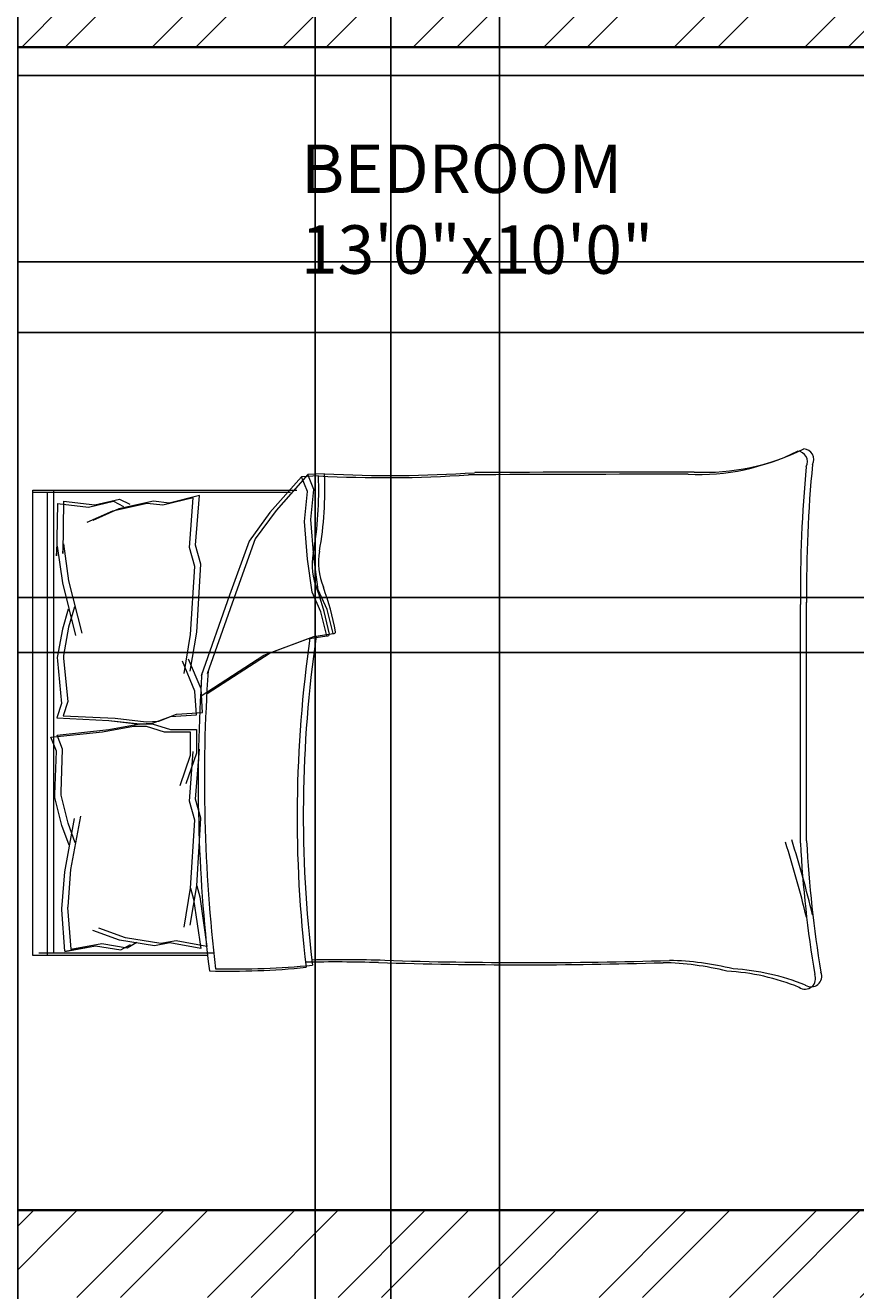
# Model space of a CAD drawing. Units: inches. Extents: x 1748 to 2382, y 1346 to 2284.
# Tile 19 of 26: x 1871 to 1956, y 1971 to 2102. Entities that reach past the tile are written whole.
import ezdxf

# ---------------------------------------------------------------- set-up
doc = ezdxf.new("R2010")
doc.units = ezdxf.units.IN
for name, color, linetype, lineweight in [('A-ANNO-DIMS', 2, 'Continuous', 18), ('A-AREA-IDEN', 7, 'Continuous', 18), ('A-FURN', 8, 'Continuous', 13), ('A-WALL', 7, 'Continuous', 35), ('A-WALL-PATT', 9, 'Continuous', 13)]:
    doc.layers.add(name, color=color, linetype=linetype, lineweight=lineweight)
doc.styles.get("Standard").update_dxf_attribs({"font": 'arial.ttf'})
doc.dimstyles.get("Standard").update_dxf_attribs({"dimtxt": 0.18, "dimasz": 0.18, "dimexe": 0.18, "dimexo": 0.0625, "dimgap": 0.09, "dimtad": 0, "dimtih": 1, "dimtoh": 1, "dimdec": 4, "dimzin": 0, "dimdsep": 46, "dimtxsty": 'Standard', "dimcen": 0.09, "dimadec": 0, "dimazin": 0, "dimtfac": 1, "dimtdec": 4, "dimtofl": 0, "dimtmove": 0, "dimatfit": 3, "dimfxl": 1, "dimtolj": 1, "dimtzin": 0, "dimarcsym": 0})

# ---------------------------------------------------------------- blocks, each defined once
blk = doc.blocks.new('BED-DOUBLE')
for p, q in [((3.48, 63.33), (3.48, 81.44)), ((3.48, 63.33), (3.48, 81.44)), ((3.48, 81.44), (51.49, 81.44)), ((51.27, 81.44), (51.27, 54.83)), ((51.27, 81.44), (51.27, 54.83)), ((51.49, 81.44), (51.49, 80.8)), ((3.48, 79.91), (51.27, 79.91)), ((3.48, 79.91), (51.27, 79.91)), ((3.7, 62.69), (3.7, 80.8)), ((3.7, 62.69), (3.7, 80.8)), ((51.49, 80.8), (51.49, 54.19)), ((51.49, 80.8), (51.49, 54.19)), ((3.7, 79.27), (51.49, 79.27)), ((3.7, 79.27), (51.49, 79.27)), ((3.9, 78.11), (8.18, 78.43)), ((3.9, 78.11), (8.18, 78.43)), ((8.18, 78.43), (8.29, 78.42)), ((8.18, 78.43), (8.28, 78.42)), ((8.28, 78.42), (12.11, 78.13)), ((8.29, 78.42), (12.11, 78.13)), ((14.86, 77.69), (16.88, 78.42)), ((14.86, 77.69), (16.88, 78.42)), ((16.88, 78.42), (19.77, 79.14)), ((16.88, 78.42), (19.77, 79.14)), ((17.11, 77.78), (20, 78.5)), ((17.11, 77.78), (20, 78.5)), ((19.77, 79.14), (20.09, 79.14)), ((19.77, 79.14), (20.09, 79.14)), ((20, 78.5), (20.32, 78.5)), ((20, 78.5), (20.32, 78.5)), ((20.09, 79.14), (24.54, 78.99)), ((20.09, 79.14), (24.54, 78.99)), ((20.32, 78.5), (24.77, 78.36)), ((20.32, 78.5), (24.77, 78.36)), ((24.54, 78.99), (25.98, 79.57)), ((24.54, 78.99), (25.98, 79.57)), ((24.77, 78.36), (26.21, 78.93)), ((24.77, 78.36), (26.21, 78.93)), ((25.98, 79.57), (26.56, 74.22)), ((25.98, 79.57), (26.56, 74.22)), ((26.21, 78.93), (26.79, 73.58)), ((26.21, 78.93), (26.79, 73.58)), ((27.98, 78.95), (27.73, 73.58)), ((27.98, 78.95), (27.73, 73.58)), ((29.46, 78.46), (27.98, 78.95)), ((29.46, 78.46), (27.98, 78.95)), ((33.88, 78.89), (29.46, 78.46)), ((33.88, 78.89), (29.46, 78.46)), ((34.21, 78.91), (33.88, 78.89)), ((34.2, 78.91), (33.88, 78.89)), ((37.14, 78.37), (34.2, 78.91)), ((37.14, 78.37), (34.21, 78.91)), ((41.91, 78.37), (36.5, 77.02)), ((41.91, 78.37), (36.5, 77.02)), ((39.2, 77.77), (37.14, 78.37)), ((39.2, 77.77), (37.14, 78.37)), ((45.71, 78.9), (41.91, 78.37)), ((45.71, 78.9), (41.91, 78.37)), ((50.11, 78.89), (44.71, 78.98)), ((44.71, 78.98), (45.71, 78.9)), ((50.11, 78.89), (44.71, 78.98)), ((44.71, 78.98), (45.71, 78.9)), ((50.34, 78.25), (44.94, 78.34)), ((44.94, 78.34), (45.94, 78.26)), ((50.34, 78.25), (44.94, 78.34)), ((44.94, 78.34), (45.94, 78.26)), ((50.11, 78.89), (49.73, 75.68)), ((50.11, 78.89), (49.73, 75.68)), ((3.89, 78.13), (4.47, 74.95)), ((3.9, 78.13), (4.47, 74.95)), ((4.12, 77.49), (4.7, 74.31)), ((4.12, 77.49), (4.7, 74.31)), ((4.13, 77.47), (8.41, 77.8)), ((4.13, 77.47), (8.41, 77.8)), ((8.41, 77.8), (8.51, 77.78)), ((8.41, 77.8), (8.51, 77.78)), ((8.51, 77.78), (12.34, 77.49)), ((8.51, 77.78), (12.34, 77.49)), ((12.11, 78.13), (17.6, 77.12)), ((12.11, 78.13), (17.6, 77.12)), ((12.34, 77.49), (17.83, 76.48)), ((12.34, 77.49), (17.83, 76.48)), ((15.08, 77.05), (17.11, 77.78)), ((15.08, 77.05), (17.11, 77.78)), ((28.21, 78.31), (27.96, 72.94)), ((28.21, 78.31), (27.96, 72.94)), ((29.68, 77.83), (28.21, 78.31)), ((29.68, 77.83), (28.21, 78.31)), ((34.11, 78.25), (29.68, 77.83)), ((34.11, 78.25), (29.68, 77.83)), ((34.43, 78.27), (34.11, 78.25)), ((34.43, 78.27), (34.11, 78.25)), ((37.36, 77.73), (34.43, 78.27)), ((37.36, 77.73), (34.43, 78.27)), ((42.14, 77.73), (36.72, 76.38)), ((42.14, 77.73), (36.72, 76.38)), ((39.43, 77.13), (37.36, 77.73)), ((39.43, 77.13), (37.36, 77.73)), ((45.94, 78.26), (42.14, 77.73)), ((45.94, 78.26), (42.14, 77.73)), ((50.34, 78.25), (49.96, 75.04)), ((50.34, 78.25), (49.96, 75.04)), ((49.31, 73.19), (48.13, 75.87)), ((49.31, 73.19), (48.13, 75.87)), ((4.47, 74.95), (4.04, 72.34)), ((4.47, 74.95), (4.04, 72.34)), ((5.05, 72.49), (6.06, 75.24)), ((5.05, 72.49), (6.06, 75.24)), ((5.28, 71.85), (6.29, 74.6)), ((5.28, 71.85), (6.29, 74.6)), ((49.54, 72.55), (48.36, 75.23)), ((49.54, 72.55), (48.36, 75.23)), ((49.73, 75.68), (50.33, 73.11)), ((49.73, 75.68), (50.33, 73.11)), ((49.96, 75.04), (50.56, 72.47)), ((49.96, 75.04), (50.56, 72.47)), ((4.7, 74.31), (4.27, 71.7)), ((4.7, 74.31), (4.27, 71.7)), ((26.56, 74.22), (27.14, 71.04)), ((26.56, 74.22), (27.14, 71.04)), ((26.79, 73.58), (27.37, 70.4)), ((26.79, 73.58), (27.37, 70.4)), ((27.73, 73.58), (27.35, 70.37)), ((27.73, 73.58), (27.36, 70.37)), ((50.11, 69.61), (49.31, 73.19)), ((50.11, 69.61), (49.31, 73.19)), ((4.04, 72.34), (4.62, 71.33)), ((4.04, 72.34), (4.62, 71.33)), ((4.47, 68.87), (5.05, 72.49)), ((4.47, 68.87), (5.05, 72.49)), ((4.7, 68.23), (5.28, 71.85)), ((4.7, 68.23), (5.28, 71.85)), ((27.96, 72.94), (27.58, 69.73)), ((27.96, 72.94), (27.58, 69.73)), ((50.34, 68.98), (49.54, 72.55)), ((50.34, 68.98), (49.54, 72.55)), ((50.33, 73.11), (49.81, 72.06)), ((50.33, 73.11), (49.81, 72.06)), ((50.56, 72.47), (50.04, 71.42)), ((50.56, 72.47), (50.04, 71.42)), ((4.27, 71.7), (4.85, 70.69)), ((4.27, 71.7), (4.85, 70.69)), ((27.14, 71.04), (27.14, 69.74)), ((27.14, 71.04), (27.14, 69.74)), ((27.14, 69.74), (26.56, 67.86)), ((27.14, 69.74), (26.56, 67.86)), ((27.35, 70.37), (27.44, 69.07)), ((27.36, 70.37), (27.44, 69.07)), ((27.37, 70.4), (27.37, 69.1)), ((27.37, 70.4), (27.37, 69.1)), ((27.58, 69.73), (27.66, 68.43)), ((27.58, 69.73), (27.66, 68.43)), ((49.92, 68.01), (50.11, 69.61)), ((49.92, 68.01), (50.11, 69.61)), ((4.76, 67.28), (4.47, 68.87)), ((4.76, 67.28), (4.47, 68.87)), ((4.99, 66.64), (4.7, 68.23)), ((4.99, 66.64), (4.7, 68.23)), ((27.37, 69.1), (26.79, 67.22)), ((27.37, 69.1), (26.79, 67.22)), ((27.44, 69.07), (28.13, 67.23)), ((27.44, 69.07), (28.13, 67.23)), ((27.66, 68.43), (28.36, 66.59)), ((27.66, 68.43), (28.36, 66.59)), ((50.7, 64.87), (49.92, 68.01)), ((50.7, 64.87), (49.92, 68.01)), ((50.15, 67.37), (50.34, 68.98)), ((50.15, 67.37), (50.34, 68.98)), ((4.18, 64.1), (4.76, 67.28)), ((4.18, 64.1), (4.76, 67.28)), ((4.41, 63.46), (4.99, 66.64)), ((4.41, 63.46), (4.99, 66.64)), ((26.56, 67.86), (26.56, 65.18)), ((26.56, 67.86), (26.56, 65.18)), ((26.79, 67.22), (26.79, 64.54)), ((26.79, 67.22), (26.79, 64.54)), ((28.13, 67.23), (28.3, 64.55)), ((28.13, 67.23), (28.3, 64.55)), ((28.36, 66.59), (28.53, 63.91)), ((28.36, 66.59), (28.53, 63.91)), ((50.93, 64.23), (50.15, 67.37)), ((50.93, 64.23), (50.15, 67.37)), ((6.38, 65.81), (10.41, 65.15)), ((6.38, 65.81), (10.41, 65.15)), ((24.1, 65.18), (20.96, 66.27)), ((24.1, 65.18), (20.96, 66.27)), ((24.33, 64.54), (21.19, 65.63)), ((24.33, 64.54), (21.19, 65.63)), ((30.75, 64.7), (33.82, 65.99)), ((30.75, 64.7), (33.82, 65.99)), ((30.98, 64.06), (34.05, 65.35)), ((30.98, 64.06), (34.05, 65.35)), ((32.56, 65.81), (36.6, 65.15)), ((32.56, 65.81), (36.6, 65.15)), ((9.28, 64.83), (4.18, 64.1)), ((9.28, 64.83), (4.18, 64.1)), ((9.51, 64.19), (4.41, 63.46)), ((9.51, 64.19), (4.41, 63.46)), ((6.61, 65.18), (10.64, 64.51)), ((6.61, 65.18), (10.64, 64.51)), ((10.41, 65.15), (9.28, 64.83)), ((10.41, 65.15), (9.28, 64.83)), ((10.64, 64.51), (9.51, 64.19)), ((10.64, 64.51), (9.51, 64.19)), ((10.41, 65.15), (17.42, 64.72)), ((10.41, 65.15), (17.42, 64.72)), ((10.64, 64.51), (17.65, 64.08)), ((10.64, 64.51), (17.65, 64.08)), ((17.42, 64.72), (19.38, 65.27)), ((17.42, 64.72), (19.38, 65.27)), ((17.65, 64.08), (19.61, 64.64)), ((17.65, 64.08), (19.61, 64.64)), ((19.38, 65.27), (24.52, 64.87)), ((19.38, 65.27), (24.52, 64.87)), ((19.61, 64.64), (24.74, 64.23)), ((19.61, 64.64), (24.74, 64.23)), ((26.56, 65.18), (24.1, 65.18)), ((26.56, 65.18), (24.1, 65.18)), ((26.79, 64.54), (24.33, 64.54)), ((26.79, 64.54), (24.33, 64.54)), ((28.3, 64.55), (30.75, 64.7)), ((28.3, 64.55), (30.75, 64.7)), ((28.53, 63.91), (30.98, 64.06)), ((28.53, 63.91), (30.98, 64.06)), ((30.26, 64.06), (34.45, 57.57)), ((30.26, 64.06), (34.45, 57.57)), ((40.64, 61.13), (32.31, 64.06)), ((40.64, 61.13), (32.31, 64.06)), ((32.79, 65.18), (36.83, 64.51)), ((32.79, 65.18), (36.82, 64.51)), ((36.6, 65.15), (43.61, 64.72)), ((36.6, 65.15), (43.61, 64.72)), ((36.82, 64.51), (43.83, 64.08)), ((36.83, 64.51), (43.83, 64.08)), ((43.61, 64.72), (45.57, 65.27)), ((43.61, 64.72), (45.57, 65.27)), ((43.83, 64.08), (45.8, 64.64)), ((43.83, 64.08), (45.79, 64.64)), ((45.57, 65.27), (50.7, 64.87)), ((45.57, 65.27), (50.7, 64.87)), ((45.79, 64.64), (50.93, 64.23)), ((45.8, 64.64), (50.93, 64.23)), ((30.49, 63.42), (34.68, 56.93)), ((30.49, 63.42), (34.68, 56.93)), ((40.87, 60.49), (32.53, 63.42)), ((40.87, 60.49), (32.53, 63.42)), ((46.22, 59.11), (40.64, 61.13)), ((46.22, 59.11), (40.64, 61.13)), ((46.45, 58.48), (40.87, 60.49)), ((46.45, 58.48), (40.87, 60.49)), ((49.16, 56.95), (46.22, 59.11)), ((49.16, 56.95), (46.22, 59.11)), ((34.45, 57.57), (36.15, 53.08)), ((34.45, 57.57), (36.15, 53.08)), ((49.39, 56.31), (46.45, 58.48)), ((49.39, 56.31), (46.45, 58.48)), ((34.68, 56.93), (36.38, 52.44)), ((34.68, 56.93), (36.38, 52.44)), ((52.87, 53.7), (49.16, 56.95)), ((52.87, 53.7), (49.16, 56.95)), ((53.1, 53.06), (49.39, 56.31)), ((53.1, 53.06), (49.39, 56.31)), ((51.33, 53.08), (52.87, 53.7)), ((51.33, 53.08), (52.87, 53.7)), ((52.95, 51.95), (52.87, 53.7, 3.87)), ((52.95, 51.95), (52.87, 53.7, 3.87)), ((36.15, 53.08), (36.46, 51.07)), ((36.15, 53.08), (36.46, 51.07)), ((36.38, 52.44), (36.69, 50.43)), ((36.38, 52.44), (36.69, 50.43)), ((38.94, 51.69), (40.95, 52.61)), ((38.94, 51.69), (40.95, 52.61)), ((40.95, 52.61), (44.36, 53.08)), ((40.95, 52.61), (44.36, 53.08)), ((41.18, 51.97), (44.59, 52.44)), ((41.18, 51.97), (44.59, 52.44)), ((44.36, 53.08), (48.23, 53.39)), ((44.36, 53.08), (48.23, 53.39)), ((44.59, 52.44), (48.46, 52.75)), ((44.59, 52.44), (48.46, 52.75)), ((48.23, 53.39), (51.33, 53.08)), ((48.23, 53.39), (51.33, 53.08)), ((48.46, 52.75), (51.56, 52.44)), ((48.46, 52.75), (51.56, 52.44)), ((51.56, 52.44), (53.1, 53.06)), ((51.56, 52.44), (53.1, 53.06)), ((53.18, 51.31), (53.1, 53.06, 3.87)), ((53.18, 51.31), (53.1, 53.06, 3.87)), ((36.46, 51.07), (38.94, 51.69)), ((36.46, 51.07), (38.94, 51.69)), ((36.69, 50.43), (39.17, 51.05)), ((36.69, 50.43), (39.17, 51.05)), ((39.17, 51.05), (41.18, 51.97)), ((39.17, 51.05), (41.18, 51.97)), ((15.06, 2.2), (39.68, 2.2)), ((15.06, 2.2), (39.68, 2.2)), ((15.29, 1.56), (39.91, 1.56)), ((15.29, 1.56), (39.91, 1.56))]:
    blk.add_line(p, q)
for centre, radius, start, end in [((21.36, -100.61), 164.97, 86.0865, 96.7821), ((21.36, -100.61), 164.97, 86.0865, 96.7821), ((85.16, 61.35), 83.31, 178.7218, 185.604), ((85.16, 61.35), 83.31, 178.7218, 185.604), ((21.59, -101.25), 164.97, 86.0865, 96.7821), ((21.59, -101.25), 164.97, 86.0865, 96.7821), ((85.39, 60.71), 83.31, 178.7218, 185.604), ((85.39, 60.71), 83.31, 178.7218, 185.604), ((17.76, -74.87), 129.02, 81.7845, 96.9006), ((17.76, -74.87), 129.02, 81.7845, 96.9006), ((17.98, -75.51), 129.02, 81.7845, 96.9006), ((17.98, -75.51), 129.02, 81.7845, 96.9006), ((-167.31, 50.27), 170.11, 358.4762, 1.0082), ((-167.31, 50.27), 170.11, 358.4762, 1.0082), ((-167.08, 49.63), 170.11, 358.4762, 1.0082), ((-167.08, 49.63), 170.11, 358.4762, 1.0082), ((43.74, 46.38), 6.22, 78.6608, 113.7384), ((43.74, 46.38), 6.22, 78.6608, 113.7384), ((51.33, 88.1), 36.18, 259.8763, 272.5657), ((51.33, 88.1), 36.18, 259.8763, 272.5657), ((36.64, 51), 0.185, 160.2464, 271.1377), ((36.64, 51), 0.185, 160.2464, 271.1377), ((31.15, 79.96), 29.65, 280.6617, 289.8806), ((31.15, 79.96), 29.65, 280.6617, 289.8806), ((31.38, 79.32), 29.65, 280.6617, 289.8806), ((31.38, 79.32), 29.65, 280.6617, 289.8806), ((43.97, 45.74), 6.22, 78.6608, 113.7384), ((43.97, 45.74), 6.22, 78.6608, 113.7384), ((51.56, 87.46), 36.18, 259.8763, 272.5657), ((51.56, 87.46), 36.18, 259.8763, 272.5657), ((182.27, 45.13), 129.5, 176.9791, 183.8365), ((182.27, 45.13), 129.5, 176.9791, 183.8365), ((182.49, 44.49), 129.5, 176.9791, 183.8365), ((182.49, 44.49), 129.5, 176.9791, 183.8365), ((36.87, 50.36), 0.185, 160.2464, 271.1377), ((36.86, 50.36), 0.185, 160.2464, 271.1377), ((484.82, 30.83), 482.31, 178.2277, 181.7185), ((484.82, 30.83), 482.31, 178.2277, 181.7185), ((485.05, 30.19), 482.31, 178.2277, 181.7185), ((485.05, 30.19), 482.31, 178.2277, 181.7185), ((-4508.74, 13.62), 4561.86, 0.00217, 0.28689), ((-4508.74, 13.62), 4561.86, 0.00217, 0.28689), ((-4508.51, 12.98), 4561.86, 0.00217, 0.28689), ((-4508.51, 12.98), 4561.86, 0.00217, 0.28689), ((-26.9, 16.93), 29.63, 346.0648, 358.9113), ((-26.9, 16.93), 29.63, 346.0648, 358.9113), ((-26.67, 16.29), 29.63, 346.0648, 358.9113), ((-26.67, 16.29), 29.63, 346.0648, 358.9113), ((76.16, 12.78), 23.07, 177.4714, 206.4681), ((76.16, 12.78), 23.07, 177.4714, 206.4681), ((76.39, 12.14), 23.07, 177.4714, 206.4681), ((76.39, 12.14), 23.07, 177.4714, 206.4681), ((-21.66, 11.17), 23.56, 337.9751, 356.652), ((-21.66, 11.17), 23.56, 337.9751, 356.652), ((-21.43, 10.53), 23.56, 337.9751, 356.652), ((-21.43, 10.53), 23.56, 337.9751, 356.652), ((-17.22, 105.16), 106.46, 283.3832, 287.7053), ((-17.22, 105.16), 106.46, 283.3832, 287.7053), ((-16.99, 104.52), 106.46, 283.3832, 287.7053), ((-16.99, 104.52), 106.46, 283.3832, 287.7053), ((1.09, 1.73), 1.09, 146.1736, 293.4781), ((1.09, 1.73), 1.09, 146.1736, 293.4781), ((1.32, 1.09), 1.09, 146.1736, 293.4781), ((1.32, 1.09), 1.09, 146.1736, 293.4781), ((21.43, -119.39), 121.76, 92.9958, 99.4091), ((21.43, -119.39), 121.76, 92.9958, 99.4091), ((21.66, -120.03), 121.76, 92.9958, 99.4091), ((21.66, -120.03), 121.76, 92.9958, 99.4091), ((41.15, -130.83), 133.04, 84.4998, 90.6351), ((41.15, -130.83), 133.04, 84.4998, 90.6351), ((41.38, -131.47), 133.04, 84.4998, 90.6351), ((41.38, -131.47), 133.04, 84.4998, 90.6351), ((54.41, 2.57), 1.1, 242.6588, 356.02), ((54.41, 2.57), 1.1, 242.6588, 356.02), ((54.64, 1.93), 1.1, 242.6588, 356.02), ((54.64, 1.93), 1.1, 242.6588, 356.02)]:
    blk.add_arc(centre, radius, start, end)
blk = doc.blocks.new('*D50')
at = {"layer": 'A-ANNO-DIMS', "color": 0, "lineweight": -2, "transparency": 16777216}
for p, q in [((1869.96, 2223.79), (1869.96, 1360.47)), ((1908.44, 2223.79), (1908.44, 1360.47)), ((1870.14, 1360.65), (1888.81, 1360.65)), ((1908.26, 1360.65), (1889.6, 1360.65))]:
    blk.add_line(p, q, dxfattribs=at)
at = {"layer": 'A-ANNO-DIMS', "color": 0, "transparency": 16777216}
for points in [[(1870.14, 1360.68), (1870.14, 1360.62), (1869.96, 1360.65)], [(1908.26, 1360.68), (1908.26, 1360.62), (1908.44, 1360.65)]]:
    blk.add_solid(points, dxfattribs=at)
at = {"layer": 'Defpoints', "color": 0, "transparency": 16777216}
for p in [(1869.96, 2223.85), (1908.44, 2223.85), (1908.44, 1360.65)]:
    blk.add_point(p, dxfattribs=at)
at = {"layer": 'A-ANNO-DIMS', "color": 0, "transparency": 16777216, "insert": (1889.2, 1360.65), "char_height": 0.18, "attachment_point": 5}
blk.add_mtext('\\A1;38.48', dxfattribs=at)
blk = doc.blocks.new('*D57')
at = {"layer": 'A-ANNO-DIMS', "color": 0, "lineweight": -2, "transparency": 16777216}
for p, q in [((2288.4, 2099.35), (1779.88, 2099.35)), ((1780.06, 2099.17), (1780.06, 2088.46)), ((1780.06, 2077.38), (1780.06, 2088.09)), ((2288.4, 2077.2), (1779.88, 2077.2))]:
    blk.add_line(p, q, dxfattribs=at)
at = {"layer": 'A-ANNO-DIMS', "color": 0, "transparency": 16777216}
for points in [[(1780.03, 2099.17), (1780.09, 2099.17), (1780.06, 2099.35)], [(1780.03, 2077.38), (1780.09, 2077.38), (1780.06, 2077.2)]]:
    blk.add_solid(points, dxfattribs=at)
at = {"layer": 'Defpoints', "color": 0, "transparency": 16777216}
for p in [(1780.06, 2099.35), (2288.46, 2099.35), (2288.46, 2077.2)]:
    blk.add_point(p, dxfattribs=at)
at = {"layer": 'A-ANNO-DIMS', "color": 0, "transparency": 16777216, "insert": (1780.06, 2088.28), "char_height": 0.18, "attachment_point": 5}
blk.add_mtext('\\A1;22.15', dxfattribs=at)
blk = doc.blocks.new('*D63')
at = {"layer": 'A-ANNO-DIMS', "color": 0, "lineweight": -2, "transparency": 16777216}
for p, q in [((2253.72, 2042.57), (1779.88, 2042.57)), ((1780.06, 2042.39), (1780.06, 2039.92)), ((1780.06, 2037.08), (1780.06, 2039.55)), ((2253.72, 2036.9), (1779.88, 2036.9))]:
    blk.add_line(p, q, dxfattribs=at)
at = {"layer": 'A-ANNO-DIMS', "color": 0, "transparency": 16777216}
for points in [[(1780.03, 2042.39), (1780.09, 2042.39), (1780.06, 2042.57)], [(1780.03, 2037.08), (1780.09, 2037.08), (1780.06, 2036.9)]]:
    blk.add_solid(points, dxfattribs=at)
at = {"layer": 'Defpoints', "color": 0, "transparency": 16777216}
for p in [(1780.06, 2042.57), (2253.78, 2042.57), (2253.78, 2036.9)]:
    blk.add_point(p, dxfattribs=at)
at = {"layer": 'A-ANNO-DIMS', "color": 0, "transparency": 16777216, "insert": (1780.06, 2039.74), "char_height": 0.18, "attachment_point": 5}
blk.add_mtext('\\A1;5.673', dxfattribs=at)
blk = doc.blocks.new('*D64')
at = {"layer": 'A-ANNO-DIMS', "color": 0, "lineweight": -2, "transparency": 16777216}
for p, q in [((1900.64, 1476.91), (1900.64, 2274.93)), ((1900.82, 2274.75), (1909.7, 2274.75)), ((1919.5, 2274.75), (1910.62, 2274.75)), ((1919.68, 1476.91), (1919.68, 2274.93))]:
    blk.add_line(p, q, dxfattribs=at)
at = {"layer": 'A-ANNO-DIMS', "color": 0, "transparency": 16777216}
for points in [[(1900.82, 2274.78), (1900.82, 2274.72), (1900.64, 2274.75)], [(1919.5, 2274.78), (1919.5, 2274.72), (1919.68, 2274.75)]]:
    blk.add_solid(points, dxfattribs=at)
at = {"layer": 'Defpoints', "color": 0, "transparency": 16777216}
for p in [(1919.68, 2274.75), (1900.64, 1476.85), (1919.68, 1476.85)]:
    blk.add_point(p, dxfattribs=at)
at = {"layer": 'A-ANNO-DIMS', "color": 0, "transparency": 16777216, "insert": (1910.16, 2274.75), "char_height": 0.18, "attachment_point": 5}
blk.add_mtext('\\A1;19.035', dxfattribs=at)
blk = doc.blocks.new('*D76')
at = {"layer": 'A-ANNO-DIMS', "color": 0, "lineweight": -2, "transparency": 16777216}
for p, q in [((2025.9, 2096.43), (1779.88, 2096.43)), ((1780.06, 2096.25), (1780.06, 2083.35)), ((1780.06, 2070.08), (1780.06, 2082.98)), ((2025.9, 2069.9), (1779.88, 2069.9))]:
    blk.add_line(p, q, dxfattribs=at)
at = {"layer": 'A-ANNO-DIMS', "color": 0, "transparency": 16777216}
for points in [[(1780.03, 2096.25), (1780.09, 2096.25), (1780.06, 2096.43)], [(1780.03, 2070.08), (1780.09, 2070.08), (1780.06, 2069.9)]]:
    blk.add_solid(points, dxfattribs=at)
at = {"layer": 'Defpoints', "color": 0, "transparency": 16777216}
for p in [(1780.06, 2096.43), (2025.96, 2096.43), (2025.96, 2069.9)]:
    blk.add_point(p, dxfattribs=at)
at = {"layer": 'A-ANNO-DIMS', "color": 0, "transparency": 16777216, "insert": (1780.06, 2083.16), "char_height": 0.18, "attachment_point": 5}
blk.add_mtext('\\A1;26.535', dxfattribs=at)

msp = doc.modelspace()

# ---------------------------------------------------------------- hatches: boundary and pattern name
at = {"layer": 'A-WALL-PATT'}
h = msp.add_hatch(dxfattribs=at)
h.set_pattern_fill('ANSI32', color=256)
h.paths.add_polyline_path([(1908.4445, 2232.8497), (1821.9607, 2232.8497), (1821.9607, 2223.8497), (1865.4607, 2223.8497), (1865.4607, 2209.9185), (1869.9607, 2209.9185), (1869.9607, 2223.8497), (1908.4445, 2223.8497), (1908.4445, 2228.3497)])
h.paths.add_polyline_path([(2040.0683, 2232.8497), (1968.4445, 2232.8497), (1968.4445, 2223.8497), (2025.9607, 2223.8497), (2025.9607, 2130.3497), (2032.1341, 2130.3497), (2032.1341, 2132.5997), (2032.1341, 2134.8497), (2030.4607, 2134.8497), (2030.4607, 2223.8497), (2040.0683, 2223.8497)])
h.paths.add_polyline_path([(2091.3969, 2232.8497), (2064.0683, 2232.8497), (2064.0683, 2223.8497), (2078.4607, 2223.8497), (2078.4607, 2134.8497), (2051.1563, 2134.8497), (2051.1563, 2130.3497), (2078.4607, 2130.3497), (2078.4607, 2128.6813), (2082.9607, 2128.6813), (2082.9607, 2130.3497), (2086.1879, 2130.3497), (2086.1879, 2132.5997), (2086.1879, 2134.8497), (2082.9607, 2134.8497), (2082.9607, 2223.8497), (2091.3969, 2223.8497), (2091.3969, 2228.3497)])
h.paths.add_polyline_path([(2167.0164, 2232.8497), (2115.3969, 2232.8497), (2115.3969, 2223.8497), (2130.9607, 2223.8497), (2130.9607, 2134.8497), (2106.9607, 2134.8497), (2106.9607, 2130.3497), (2135.4607, 2130.3497), (2135.4607, 2223.8497), (2167.0164, 2223.8497), (2167.0164, 2228.3497)])
h.paths.add_polyline_path([(1869.9607, 2149.9185), (1865.4607, 2149.9185), (1865.4607, 2127.8942), (1869.9607, 2127.8942)])
h.paths.add_polyline_path([(2082.9607, 2104.4871), (2080.7107, 2104.4871), (2078.4607, 2104.4871), (2078.4607, 2103.8497), (1869.9607, 2103.8497), (1869.9607, 2108.6062), (1867.7107, 2108.6062), (1865.4607, 2108.6062), (1865.4607, 2103.8497), (1821.9607, 2103.8497), (1821.9607, 2099.3497), (1865.4607, 2099.3497), (1865.4607, 2094.7509), (1869.9607, 2094.7509), (1869.9607, 2099.3497), (2025.9607, 2099.3497), (2025.9607, 2096.4326), (2030.4607, 2096.4326), (2030.4607, 2099.3497), (2082.9607, 2099.3497)])
h.paths.add_polyline_path([(1928.9457, 1401.1212), (2176.8693, 1401.1212), (2176.8693, 1438.214), (1928.9457, 1438.214)], flags=9)
h.paths.add_polyline_path([(2122.2668, 2048.1927), (2177.9387, 2048.1927), (2177.9387, 2066.85), (2122.2668, 2066.85)], flags=9)
h.paths.add_polyline_path([(2272.688, 2153.8197), (2272.688, 2216.746), (2262.3845, 2216.746), (2262.3845, 2153.8197)], flags=9)
h.paths.add_polyline_path([(2157.2928, 2166.5593), (2196.3822, 2166.5593), (2196.3822, 2185.2167), (2157.2928, 2185.2167)], flags=9)
h.paths.add_polyline_path([(2089.3407, 2162.0698), (2124.3987, 2162.0698), (2124.3987, 2180.7272), (2089.3407, 2180.7272)], flags=9)
h.paths.add_polyline_path([(2037.4521, 2160.0913), (2072.5101, 2160.0913), (2072.5101, 2178.7486), (2037.4521, 2178.7486)], flags=9)
h.paths.add_polyline_path([(1884.7894, 2104.1554), (1923.6297, 2104.1554), (1923.6297, 2122.8127), (1884.7894, 2122.8127)], flags=9)
h.paths.add_polyline_path([(1851.2832, 2142.9749), (1851.2832, 2199.3051), (1840.9796, 2199.3051), (1840.9796, 2142.9749)], flags=9)
h.paths.add_polyline_path([(1844.8763, 2017.2834), (1844.8763, 2073.6136), (1834.5728, 2073.6136), (1834.5728, 2017.2834)], flags=9)
h.paths.add_polyline_path([(1897.1577, 2073.1279), (1935.9981, 2073.1279), (1935.9981, 2091.7853), (1897.1577, 2091.7853)], flags=9)
h.paths.add_polyline_path([(1952.3395, 1802.4231), (2008.0114, 1802.4231), (2008.0114, 1821.0805), (1952.3395, 1821.0805)], flags=9)
h.paths.add_polyline_path([(1978.8184, 1857.6841), (2017.7338, 1857.6841), (2017.7338, 1876.3415), (1978.8184, 1876.3415)], flags=9)
h.paths.add_polyline_path([(1979.6513, 1925.9516), (2008.8089, 1925.9516), (2008.8089, 1944.6089), (1979.6513, 1944.6089)], flags=9)
h.paths.add_polyline_path([(1838.5553, 1860.3527), (1877.3957, 1860.3527), (1877.3957, 1879.01), (1838.5553, 1879.01)], flags=9)
h.paths.add_polyline_path([(1883.9018, 1787.3013), (1883.9018, 1843.6315), (1873.5983, 1843.6315), (1873.5983, 1787.3013)], flags=9)
h.paths.add_polyline_path([(1873.7079, 1509.1938), (1873.7079, 1583.7709), (1863.4044, 1583.7709), (1863.4044, 1509.1938)], flags=9)
h.paths.add_polyline_path([(1916.2259, 1603.3681), (1955.0663, 1603.3681), (1955.0663, 1622.0254), (1916.2259, 1622.0254)], flags=9)
h.paths.add_polyline_path([(1876.3013, 1636.757), (1876.3013, 1693.0871), (1865.9978, 1693.0871), (1865.9978, 1636.757)], flags=9)
h.paths.add_polyline_path([(1921.3138, 1521.8316), (1964.0662, 1521.8316), (1964.0662, 1540.489), (1921.3138, 1540.489)], flags=9)
h.paths.add_polyline_path([(2017.5657, 1497.5078), (2046.7983, 1497.5078), (2046.7983, 1516.1651), (2017.5657, 1516.1651)], flags=9)
h.paths.add_polyline_path([(2066.8661, 1499.3902), (2096.0988, 1499.3902), (2096.0988, 1518.0475), (2066.8661, 1518.0475)], flags=9)
h.paths.add_polyline_path([(2155.4835, 1571.6596), (2198.2358, 1571.6596), (2198.2358, 1590.3169), (2155.4835, 1590.3169)], flags=9)
h.paths.add_polyline_path([(2094.9136, 1664.6812), (2150.5855, 1664.6812), (2150.5855, 1683.3386), (2094.9136, 1683.3386)], flags=9)
h.paths.add_polyline_path([(2257.6902, 1863.1628), (2269.8935, 1863.1628), (2269.8935, 1873.4664), (2257.6902, 1873.4664)], flags=9)
h.paths.add_polyline_path([(2164.0748, 1880.3089), (2189.8694, 1880.3089), (2189.8694, 1890.6124), (2164.0748, 1890.6124)], flags=9)
h.paths.add_polyline_path([(2239.4394, 1931.0585), (2268.8187, 1931.0585), (2268.8187, 1949.7159), (2239.4394, 1949.7159)], flags=9)
h = msp.add_hatch(dxfattribs=at)
h.set_pattern_fill('ANSI32', color=256)
h.paths.add_polyline_path([(2297.4607, 2232.8497), (2203.0164, 2232.8497), (2203.0164, 2223.8497), (2244.9607, 2223.8497), (2244.9607, 2127.8554), (2249.4607, 2127.8554), (2249.4607, 2223.8497), (2297.4607, 2223.8497)])
h.paths.add_polyline_path([(2297.4607, 2103.8497), (2249.4607, 2103.8497), (2249.4607, 2106.7497), (2247.2107, 2106.7497), (2244.9607, 2106.7497), (2244.9607, 2103.8497), (2130.9607, 2103.8497), (2130.9607, 2099.3497), (2288.4607, 2099.3497), (2288.4607, 2077.2008), (2297.4607, 2077.2008)])
h.paths.add_polyline_path([(1928.9457, 1401.1212), (2176.8693, 1401.1212), (2176.8693, 1438.214), (1928.9457, 1438.214)], flags=9)
h.paths.add_polyline_path([(2122.2668, 2048.1927), (2177.9387, 2048.1927), (2177.9387, 2066.85), (2122.2668, 2066.85)], flags=9)
h.paths.add_polyline_path([(2272.688, 2153.8197), (2272.688, 2216.746), (2262.3845, 2216.746), (2262.3845, 2153.8197)], flags=25)
h.paths.add_polyline_path([(2157.2928, 2166.5593), (2196.3822, 2166.5593), (2196.3822, 2185.2167), (2157.2928, 2185.2167)], flags=9)
h.paths.add_polyline_path([(2089.3407, 2162.0698), (2124.3987, 2162.0698), (2124.3987, 2180.7272), (2089.3407, 2180.7272)], flags=9)
h.paths.add_polyline_path([(2037.4521, 2160.0913), (2072.5101, 2160.0913), (2072.5101, 2178.7486), (2037.4521, 2178.7486)], flags=9)
h.paths.add_polyline_path([(1884.7894, 2104.1554), (1923.6297, 2104.1554), (1923.6297, 2122.8127), (1884.7894, 2122.8127)], flags=9)
h.paths.add_polyline_path([(1851.2832, 2142.9749), (1851.2832, 2199.3051), (1840.9796, 2199.3051), (1840.9796, 2142.9749)], flags=9)
h.paths.add_polyline_path([(1844.8763, 2017.2834), (1844.8763, 2073.6136), (1834.5728, 2073.6136), (1834.5728, 2017.2834)], flags=9)
h.paths.add_polyline_path([(1897.1577, 2073.1279), (1935.9981, 2073.1279), (1935.9981, 2091.7853), (1897.1577, 2091.7853)], flags=9)
h.paths.add_polyline_path([(1952.3395, 1802.4231), (2008.0114, 1802.4231), (2008.0114, 1821.0805), (1952.3395, 1821.0805)], flags=9)
h.paths.add_polyline_path([(1978.8184, 1857.6841), (2017.7338, 1857.6841), (2017.7338, 1876.3415), (1978.8184, 1876.3415)], flags=9)
h.paths.add_polyline_path([(1979.6513, 1925.9516), (2008.8089, 1925.9516), (2008.8089, 1944.6089), (1979.6513, 1944.6089)], flags=9)
h.paths.add_polyline_path([(1838.5553, 1860.3527), (1877.3957, 1860.3527), (1877.3957, 1879.01), (1838.5553, 1879.01)], flags=9)
h.paths.add_polyline_path([(1883.9018, 1787.3013), (1883.9018, 1843.6315), (1873.5983, 1843.6315), (1873.5983, 1787.3013)], flags=9)
h.paths.add_polyline_path([(1873.7079, 1509.1938), (1873.7079, 1583.7709), (1863.4044, 1583.7709), (1863.4044, 1509.1938)], flags=9)
h.paths.add_polyline_path([(1916.2259, 1603.3681), (1955.0663, 1603.3681), (1955.0663, 1622.0254), (1916.2259, 1622.0254)], flags=9)
h.paths.add_polyline_path([(1876.3013, 1636.757), (1876.3013, 1693.0871), (1865.9978, 1693.0871), (1865.9978, 1636.757)], flags=9)
h.paths.add_polyline_path([(1921.3138, 1521.8316), (1964.0662, 1521.8316), (1964.0662, 1540.489), (1921.3138, 1540.489)], flags=9)
h.paths.add_polyline_path([(2017.5657, 1497.5078), (2046.7983, 1497.5078), (2046.7983, 1516.1651), (2017.5657, 1516.1651)], flags=9)
h.paths.add_polyline_path([(2066.8661, 1499.3902), (2096.0988, 1499.3902), (2096.0988, 1518.0475), (2066.8661, 1518.0475)], flags=9)
h.paths.add_polyline_path([(2155.4835, 1571.6596), (2198.2358, 1571.6596), (2198.2358, 1590.3169), (2155.4835, 1590.3169)], flags=9)
h.paths.add_polyline_path([(2094.9136, 1664.6812), (2150.5855, 1664.6812), (2150.5855, 1683.3386), (2094.9136, 1683.3386)], flags=9)
h.paths.add_polyline_path([(2257.6902, 1863.1628), (2269.8935, 1863.1628), (2269.8935, 1873.4664), (2257.6902, 1873.4664)], flags=9)
h.paths.add_polyline_path([(2164.0748, 1880.3089), (2189.8694, 1880.3089), (2189.8694, 1890.6124), (2164.0748, 1890.6124)], flags=9)
h.paths.add_polyline_path([(2239.4394, 1931.0585), (2268.8187, 1931.0585), (2268.8187, 1949.7159), (2239.4394, 1949.7159)], flags=9)
h = msp.add_hatch(dxfattribs=at)
h.set_pattern_fill('ANSI32', color=256)
h.paths.add_polyline_path([(1919.6777, 1476.8497), (1900.6426, 1476.8497), (1900.6426, 1522.0826), (1898.3926, 1522.0826), (1896.1426, 1522.0826), (1896.1426, 1476.8497), (1857.1426, 1476.8497), (1857.1426, 1467.8497), (1896.1426, 1467.8497), (1919.6777, 1467.8497), (1919.6777, 1472.3497)])
h.paths.add_polyline_path([(2018.7873, 1472.3497), (2018.7873, 1476.8497), (2010.9607, 1476.8497), (2010.9607, 1560.8497), (2034.9607, 1560.8497), (2034.9607, 1565.3497), (2006.4607, 1565.3497), (2006.4607, 1476.8497), (1955.6777, 1476.8497), (1955.6777, 1467.8497), (2018.7873, 1467.8497)])
h.paths.add_polyline_path([(2152.3354, 1472.3497), (2152.3354, 1476.8497), (2115.9607, 1476.8497), (2115.9607, 1565.3497), (2109.2204, 1565.3497), (2109.2204, 1563.0997), (2109.2204, 1560.8497), (2111.4607, 1560.8497), (2111.4607, 1476.8497), (2095.3617, 1476.8497), (2095.3617, 1467.8497), (2152.3354, 1467.8497)])
h.paths.add_polyline_path([(2071.3617, 1476.8497), (2063.4607, 1476.8497), (2063.4607, 1560.8497), (2090.1865, 1560.8497), (2090.1865, 1565.3497), (2063.4607, 1565.3497), (2063.4607, 1572.5485), (2061.2107, 1572.5485), (2058.9607, 1572.5485), (2058.9607, 1565.3497), (2055.6281, 1565.3497), (2055.6281, 1560.8497), (2058.9607, 1560.8497), (2058.9607, 1476.8497), (2042.7873, 1476.8497), (2042.7873, 1467.8497), (2071.3617, 1467.8497), (2071.3617, 1472.3497)])
h.paths.add_polyline_path([(2297.4607, 1506.5652), (2288.4607, 1506.5652), (2288.4607, 1476.8497), (2212.3354, 1476.8497), (2212.3354, 1467.8497), (2297.4607, 1467.8497)])
h.paths.add_polyline_path([(2297.4607, 1645.3038), (2288.4607, 1645.3038), (2288.4607, 1605.8497), (2058.9607, 1605.8497), (2058.9607, 1600.1857), (2061.2107, 1600.1857), (2063.4607, 1600.1857), (2063.4607, 1601.3497), (2288.4607, 1601.3497), (2288.4607, 1566.5652), (2297.4607, 1566.5652)])
h.paths.add_polyline_path([(2010.9607, 1609.0561), (2008.7107, 1609.0561), (2006.4607, 1609.0561), (2006.4607, 1605.8497), (1900.6426, 1605.8497), (1900.6426, 1609.7171), (1898.3926, 1609.7171), (1896.1426, 1609.7171), (1896.1426, 1605.8497), (1857.1426, 1605.8497), (1857.1426, 1601.3497), (1896.1426, 1601.3497), (1896.1426, 1542.5447), (1900.6426, 1542.5447), (1900.6426, 1601.3497), (2010.9607, 1601.3497)])
h.paths.add_polyline_path([(1928.9457, 1401.1212), (2176.8693, 1401.1212), (2176.8693, 1438.214), (1928.9457, 1438.214)], flags=9)
h.paths.add_polyline_path([(2122.2668, 2048.1927), (2177.9387, 2048.1927), (2177.9387, 2066.85), (2122.2668, 2066.85)], flags=9)
h.paths.add_polyline_path([(2272.688, 2153.8197), (2272.688, 2216.746), (2262.3845, 2216.746), (2262.3845, 2153.8197)], flags=9)
h.paths.add_polyline_path([(2157.2928, 2166.5593), (2196.3822, 2166.5593), (2196.3822, 2185.2167), (2157.2928, 2185.2167)], flags=9)
h.paths.add_polyline_path([(2089.3407, 2162.0698), (2124.3987, 2162.0698), (2124.3987, 2180.7272), (2089.3407, 2180.7272)], flags=9)
h.paths.add_polyline_path([(2037.4521, 2160.0913), (2072.5101, 2160.0913), (2072.5101, 2178.7486), (2037.4521, 2178.7486)], flags=9)
h.paths.add_polyline_path([(1884.7894, 2104.1554), (1923.6297, 2104.1554), (1923.6297, 2122.8127), (1884.7894, 2122.8127)], flags=9)
h.paths.add_polyline_path([(1851.2832, 2142.9749), (1851.2832, 2199.3051), (1840.9796, 2199.3051), (1840.9796, 2142.9749)], flags=9)
h.paths.add_polyline_path([(1844.8763, 2017.2834), (1844.8763, 2073.6136), (1834.5728, 2073.6136), (1834.5728, 2017.2834)], flags=9)
h.paths.add_polyline_path([(1897.1577, 2073.1279), (1935.9981, 2073.1279), (1935.9981, 2091.7853), (1897.1577, 2091.7853)], flags=9)
h.paths.add_polyline_path([(1952.3395, 1802.4231), (2008.0114, 1802.4231), (2008.0114, 1821.0805), (1952.3395, 1821.0805)], flags=9)
h.paths.add_polyline_path([(1978.8184, 1857.6841), (2017.7338, 1857.6841), (2017.7338, 1876.3415), (1978.8184, 1876.3415)], flags=9)
h.paths.add_polyline_path([(1979.6513, 1925.9516), (2008.8089, 1925.9516), (2008.8089, 1944.6089), (1979.6513, 1944.6089)], flags=9)
h.paths.add_polyline_path([(1838.5553, 1860.3527), (1877.3957, 1860.3527), (1877.3957, 1879.01), (1838.5553, 1879.01)], flags=9)
h.paths.add_polyline_path([(1883.9018, 1787.3013), (1883.9018, 1843.6315), (1873.5983, 1843.6315), (1873.5983, 1787.3013)], flags=9)
h.paths.add_polyline_path([(1873.7079, 1509.1938), (1873.7079, 1583.7709), (1863.4044, 1583.7709), (1863.4044, 1509.1938)], flags=9)
h.paths.add_polyline_path([(1916.2259, 1603.3681), (1955.0663, 1603.3681), (1955.0663, 1622.0254), (1916.2259, 1622.0254)], flags=9)
h.paths.add_polyline_path([(1876.3013, 1636.757), (1876.3013, 1693.0871), (1865.9978, 1693.0871), (1865.9978, 1636.757)], flags=9)
h.paths.add_polyline_path([(1921.3138, 1521.8316), (1964.0662, 1521.8316), (1964.0662, 1540.489), (1921.3138, 1540.489)], flags=9)
h.paths.add_polyline_path([(2017.5657, 1497.5078), (2046.7983, 1497.5078), (2046.7983, 1516.1651), (2017.5657, 1516.1651)], flags=9)
h.paths.add_polyline_path([(2066.8661, 1499.3902), (2096.0988, 1499.3902), (2096.0988, 1518.0475), (2066.8661, 1518.0475)], flags=9)
h.paths.add_polyline_path([(2155.4835, 1571.6596), (2198.2358, 1571.6596), (2198.2358, 1590.3169), (2155.4835, 1590.3169)], flags=25)
h.paths.add_polyline_path([(2094.9136, 1664.6812), (2150.5855, 1664.6812), (2150.5855, 1683.3386), (2094.9136, 1683.3386)], flags=9)
h.paths.add_polyline_path([(2257.6902, 1863.1628), (2269.8935, 1863.1628), (2269.8935, 1873.4664), (2257.6902, 1873.4664)], flags=9)
h.paths.add_polyline_path([(2164.0748, 1880.3089), (2189.8694, 1880.3089), (2189.8694, 1890.6124), (2164.0748, 1890.6124)], flags=9)
h.paths.add_polyline_path([(2239.4394, 1931.0585), (2268.8187, 1931.0585), (2268.8187, 1949.7159), (2239.4394, 1949.7159)], flags=9)
h = msp.add_hatch(dxfattribs=at)
h.set_pattern_fill('ANSI32', color=256)
h.paths.add_polyline_path([(1900.6426, 1652.723), (1896.1426, 1652.723), (1896.1426, 1629.9029), (1900.6426, 1629.9029)])
h.paths.add_polyline_path([(2206.0699, 1859.3497), (2197.0699, 1859.3497), (2197.0699, 1734.8497), (2206.0699, 1734.8497)], flags=17)
h.paths.add_polyline_path([(2297.4607, 1865.3269), (2288.4607, 1865.3269), (2288.4607, 1734.8497), (2206.0699, 1734.8497), (2180.4551, 1734.8497), (2180.4551, 1725.8497), (2197.0699, 1725.8497), (2206.0699, 1725.8497), (2288.4607, 1725.8497), (2288.4607, 1705.3038), (2297.4607, 1705.3038)])
h.paths.add_polyline_path([(2139.9607, 1815.8001), (2135.4607, 1815.8001), (2130.9607, 1815.8001), (2130.9607, 1734.8497), (1900.6426, 1734.8497), (1900.6426, 1738.9477), (1898.3926, 1738.9477), (1896.1426, 1738.9477), (1896.1426, 1734.8497), (1857.1426, 1734.8497), (1857.1426, 1725.8497), (1896.1426, 1725.8497), (1896.1426, 1712.723), (1900.6426, 1712.723), (1900.6426, 1725.8497), (2006.4607, 1725.8497), (2006.4607, 1637.448), (2010.9607, 1637.448), (2010.9607, 1725.8497), (2139.9607, 1725.8497), (2147.389, 1725.8497), (2147.389, 1730.3497), (2147.389, 1734.8497), (2139.9607, 1734.8497)])
h.paths.add_polyline_path([(2149.8497, 1917.8497), (2149.8497, 1922.3497), (2139.9607, 1922.3497), (2139.9607, 1979.3497), (2030.4607, 1979.3497), (2030.4607, 2069.8971), (2028.2107, 2069.8971), (2025.9607, 2069.8971), (2025.9607, 1979.3497), (1869.9607, 1979.3497), (1869.9607, 1998.93), (1865.4607, 1998.93), (1865.4607, 1979.3497), (1821.9607, 1979.3497), (1821.9607, 1952.7922), (1826.9306, 1952.7922), (1830.9607, 1952.7922), (1830.9607, 1970.3497), (1962.9607, 1970.3497), (1962.9607, 1926.5713), (1967.4607, 1926.5713), (1967.4607, 1970.3497), (2027.4607, 1970.3497), (2027.4607, 1898.3497), (2004.9604, 1898.3497), (2004.9604, 1893.8497), (2027.4607, 1893.8497), (2027.4607, 1859.3497), (1958.8973, 1859.3497), (1958.8973, 1854.8497), (2047.917, 1854.8497), (2047.917, 1859.3497), (2031.9607, 1859.3497), (2031.9607, 1970.3497), (2130.9607, 1970.3497), (2130.9607, 1859.3497), (2104.9565, 1859.3497), (2104.9565, 1854.8497), (2130.9607, 1854.8497), (2130.9607, 1849.0684), (2139.9607, 1849.0684), (2139.9607, 1913.3497), (2149.8497, 1913.3497)])
h.paths.add_polyline_path([(1928.9996, 1859.3497), (1830.9607, 1859.3497), (1830.9607, 1892.7922), (1821.9607, 1892.7922), (1821.9607, 1854.8497), (1896.1426, 1854.8497), (1896.1426, 1836.6443), (1898.378, 1836.6443), (1900.6426, 1836.6443), (1900.6426, 1854.8497), (1928.9996, 1854.8497), (1928.9996, 1857.0997)])
h.paths.add_polyline_path([(1980.9604, 1896.0997), (1980.9604, 1898.3497), (1967.4607, 1898.3497), (1967.4607, 1902.3846), (1962.9607, 1902.3846), (1962.9607, 1859.3497), (1967.4607, 1859.3497), (1967.4607, 1893.8497), (1980.9604, 1893.8497)], flags=17)
h.paths.add_polyline_path([(1900.6426, 1776.6443), (1896.1426, 1776.6443), (1896.1426, 1758.0891), (1900.6426, 1758.0891)], flags=17)
h.paths.add_polyline_path([(2297.4607, 2017.2008), (2288.4607, 2017.2008), (2288.4607, 1979.3497), (2213.4607, 1979.3497), (2213.4607, 1922.3497), (2183.3516, 1922.3497), (2183.3516, 1913.3497), (2213.4607, 1913.3497), (2236.234, 1913.3497), (2236.234, 1922.3497), (2222.4607, 1922.3497), (2222.4607, 1931.3497), (2222.4607, 1970.3497), (2288.4607, 1970.3497), (2288.4607, 1922.3497), (2272.1921, 1922.3497), (2272.1921, 1913.3497), (2288.4607, 1913.3497), (2288.4607, 1901.3269), (2297.4607, 1901.3269)])

# ---------------------------------------------------------------- linework, layer by layer
at = {"layer": 'A-WALL'}
for p, q in [((1869.9607, 2099.3497), (2025.9607, 2099.3497)), ((1869.9607, 1979.3497), (2025.9607, 1979.3497))]:
    msp.add_line(p, q, dxfattribs=at)

# ---------------------------------------------------------------- block references
at = {"layer": 'A-FURN', "rotation": 90}
msp.add_blockref('BED-DOUBLE', (1952.9256, 2002.1607), dxfattribs=at)

# ---------------------------------------------------------------- texts
at = {"layer": 'A-AREA-IDEN', "insert": (1899.1682, 2089.3006), "char_height": 5, "attachment_point": 1}
msp.add_mtext_dynamic_manual_height_columns('BEDROOM\\P13\'0"x10\'0"', width=263.709135, gutter_width=12.5, heights=[0], dxfattribs=at)

# ---------------------------------------------------------------- dimensions: what is measured, and where the dimension line sits
at = {"layer": 'A-ANNO-DIMS'}
for base, p1, p2, override, picture, middle in [((1919.6777, 2274.7497), (1900.6426, 1476.8497), (1919.6777, 1476.8497), {"dimdec": 3, "dimlfac": 1, "dimrnd": 0, "dimzin": 0, "dimdsep": 46, "dimlunit": 2}, '*D64', (1910.1602, 2274.7497)), ((1908.4445, 1360.6451), (1869.9607, 2223.8497), (1908.4445, 2223.8497), {"dimdec": 2, "dimlfac": 1, "dimrnd": 0, "dimzin": 0, "dimdsep": 46, "dimlunit": 2}, '*D50', (1889.2026, 1360.6451))]:
    dim = msp.add_linear_dim(base=base, p1=p1, p2=p2, dimstyle='Standard', override=override, dxfattribs=at)
    dim.commit()
    dim.dimension.update_dxf_attribs({"geometry": picture, "text_midpoint": middle})
for base, p1, p2, override, picture, middle in [((1780.0607, 2099.3497), (2288.4607, 2077.2008), (2288.4607, 2099.3497), {"dimdec": 2, "dimlfac": 1, "dimrnd": 0, "dimzin": 0, "dimdsep": 46, "dimlunit": 2}, '*D57', (1780.0607, 2088.2752)), ((1780.06066, 2096.4326), (2025.96066, 2069.89715), (2025.96066, 2096.4326), {"dimdec": 3, "dimlfac": 1, "dimrnd": 0, "dimzin": 0, "dimdsep": 46, "dimlunit": 2}, '*D76', (1780.06066, 2083.16488)), ((1780.0607, 2042.573), (2253.7809, 2036.9), (2253.7809, 2042.573), {"dimdec": 3, "dimlfac": 1, "dimrnd": 0, "dimzin": 0, "dimdsep": 46, "dimlunit": 2}, '*D63', (1780.0607, 2039.7365))]:
    dim = msp.add_linear_dim(base=base, p1=p1, p2=p2, angle=90, dimstyle='Standard', override=override, dxfattribs=at)
    dim.commit()
    dim.dimension.update_dxf_attribs({"geometry": picture, "text_midpoint": middle})

doc.saveas('drawing.dxf')
